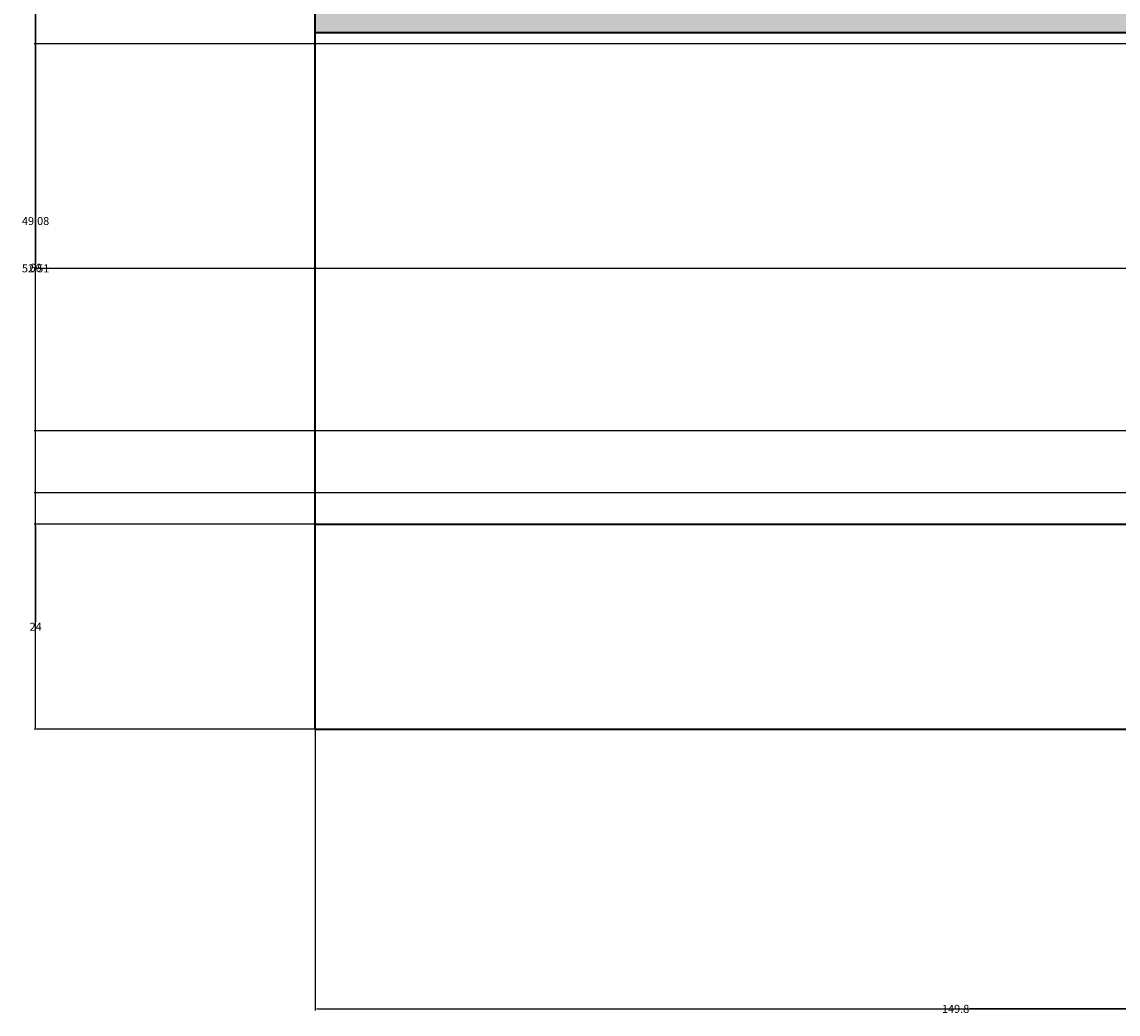
# Model space of a CAD drawing. Units: inches. Extents: x -5 to 714, y 84 to 644.
# Tile 1 of 20: x -4 to 124, y 84 to 200. Entities that reach past the tile are written whole.
import ezdxf

# ---------------------------------------------------------------- set-up
doc = ezdxf.new("R2010")
doc.units = ezdxf.units.IN
doc.header["$MEASUREMENT"] = 0
for name, color, linetype, lineweight in [('A-ANNO-DIMS', 2, 'Continuous', 18), ('A-ELEV', 7, 'Continuous', 35), ('A-ELEV-PATT', 8, 'Continuous', 13)]:
    doc.layers.add(name, color=color, linetype=linetype, lineweight=lineweight)
doc.styles.get("Standard").update_dxf_attribs({"font": 'arial.ttf'})
doc.dimstyles.get("Standard").update_dxf_attribs({"dimtxt": 0.9375, "dimasz": 0.18, "dimexe": 0.18, "dimexo": 0.0625, "dimgap": 0.09, "dimtad": 0, "dimtih": 1, "dimtoh": 1, "dimdec": 4, "dimzin": 0, "dimdsep": 46, "dimlunit": 4, "dimtxsty": 'Standard', "dimcen": 0.09, "dimadec": 0, "dimazin": 0, "dimtfac": 1, "dimtdec": 4, "dimtofl": 0, "dimtmove": 0, "dimatfit": 3, "dimfxl": 1, "dimtolj": 1, "dimtzin": 0, "dimarcsym": 0})

# ---------------------------------------------------------------- blocks, each defined once
blk = doc.blocks.new('*D1')
at = {"layer": 'A-ANNO-DIMS', "color": 0, "lineweight": -2, "transparency": 16777216}
for p, q in [((30.14, 117.13), (30.14, 84.31)), ((679.78, 117.13), (679.78, 84.31)), ((30.32, 84.49), (353.29, 84.49)), ((679.6, 84.49), (356.64, 84.49))]:
    blk.add_line(p, q, dxfattribs=at)
at = {"layer": 'A-ANNO-DIMS', "color": 0, "transparency": 16777216}
for points in [[(30.32, 84.52), (30.32, 84.46), (30.14, 84.49)], [(679.6, 84.52), (679.6, 84.46), (679.78, 84.49)]]:
    blk.add_solid(points, dxfattribs=at)
at = {"layer": 'Defpoints', "color": 0, "transparency": 16777216}
for p in [(30.14, 117.19), (679.78, 117.19), (679.78, 84.49)]:
    blk.add_point(p, dxfattribs=at)
at = {"layer": 'A-ANNO-DIMS', "color": 0, "transparency": 16777216, "insert": (354.96, 84.49), "char_height": 0.938, "attachment_point": 5}
blk.add_mtext('\\A1;649.6', dxfattribs=at)
blk = doc.blocks.new('*D2')
at = {"layer": 'A-ANNO-DIMS', "color": 0, "lineweight": -2, "transparency": 16777216}
for p, q in [((67.93, 610.73), (-2.74, 610.73)), ((-2.56, 610.55), (-2.56, 364.53)), ((-2.56, 117.37), (-2.56, 363.39)), ((30.08, 117.19), (-2.74, 117.19))]:
    blk.add_line(p, q, dxfattribs=at)
at = {"layer": 'A-ANNO-DIMS', "color": 0, "transparency": 16777216}
for points in [[(-2.59, 610.55), (-2.53, 610.55), (-2.56, 610.73)], [(-2.59, 117.37), (-2.53, 117.37), (-2.56, 117.19)]]:
    blk.add_solid(points, dxfattribs=at)
at = {"layer": 'Defpoints', "color": 0, "transparency": 16777216}
for p in [(-2.56, 610.73), (67.99, 610.73), (30.14, 117.19)]:
    blk.add_point(p, dxfattribs=at)
at = {"layer": 'A-ANNO-DIMS', "color": 0, "transparency": 16777216, "insert": (-2.56, 363.96), "char_height": 0.938, "attachment_point": 5}
blk.add_mtext('\\A1;493.5', dxfattribs=at)
blk = doc.blocks.new('*D3')
at = {"layer": 'A-ANNO-DIMS', "color": 0, "lineweight": -2, "transparency": 16777216}
for p, q in [((30.08, 141.19), (-2.74, 141.19)), ((-2.56, 141.01), (-2.56, 129.75)), ((-2.56, 117.37), (-2.56, 128.63)), ((30.08, 117.19), (-2.74, 117.19))]:
    blk.add_line(p, q, dxfattribs=at)
at = {"layer": 'A-ANNO-DIMS', "color": 0, "transparency": 16777216}
for points in [[(-2.59, 141.01), (-2.53, 141.01), (-2.56, 141.19)], [(-2.59, 117.37), (-2.53, 117.37), (-2.56, 117.19)]]:
    blk.add_solid(points, dxfattribs=at)
at = {"layer": 'Defpoints', "color": 0, "transparency": 16777216}
for p in [(-2.56, 141.19), (30.14, 141.19), (30.14, 117.19)]:
    blk.add_point(p, dxfattribs=at)
at = {"layer": 'A-ANNO-DIMS', "color": 0, "transparency": 16777216, "insert": (-2.56, 129.19), "char_height": 0.938, "attachment_point": 5}
blk.add_mtext('\\A1;24', dxfattribs=at)
blk = doc.blocks.new('*D4')
at = {"layer": 'A-ANNO-DIMS', "color": 0, "lineweight": -2, "transparency": 16777216}
for p, q in [((30.08, 201.19), (-2.74, 201.19)), ((-2.56, 201.01), (-2.56, 171.76)), ((-2.56, 141.37), (-2.56, 170.62)), ((30.08, 141.19), (-2.74, 141.19))]:
    blk.add_line(p, q, dxfattribs=at)
at = {"layer": 'A-ANNO-DIMS', "color": 0, "transparency": 16777216}
for points in [[(-2.59, 201.01), (-2.53, 201.01), (-2.56, 201.19)], [(-2.59, 141.37), (-2.53, 141.37), (-2.56, 141.19)]]:
    blk.add_solid(points, dxfattribs=at)
at = {"layer": 'Defpoints', "color": 0, "transparency": 16777216}
for p in [(-2.56, 201.19), (30.14, 201.19), (30.14, 141.19)]:
    blk.add_point(p, dxfattribs=at)
at = {"layer": 'A-ANNO-DIMS', "color": 0, "transparency": 16777216, "insert": (-2.56, 171.19), "char_height": 0.938, "attachment_point": 5}
blk.add_mtext('\\A1;60', dxfattribs=at)
blk = doc.blocks.new('*D65')
at = {"layer": 'A-ANNO-DIMS', "color": 0, "lineweight": -2, "transparency": 16777216}
for p, q in [((325.77, 266), (-2.74, 266)), ((-2.56, 265.82), (-2.56, 219.13)), ((-2.56, 171.3), (-2.56, 217.99)), ((325.77, 171.12), (-2.74, 171.12))]:
    blk.add_line(p, q, dxfattribs=at)
at = {"layer": 'A-ANNO-DIMS', "color": 0, "transparency": 16777216}
for points in [[(-2.59, 265.82), (-2.53, 265.82), (-2.56, 266)], [(-2.59, 171.3), (-2.53, 171.3), (-2.56, 171.12)]]:
    blk.add_solid(points, dxfattribs=at)
at = {"layer": 'Defpoints', "color": 0, "transparency": 16777216}
for p in [(-2.56, 266), (325.83, 266), (325.83, 171.12)]:
    blk.add_point(p, dxfattribs=at)
at = {"layer": 'A-ANNO-DIMS', "color": 0, "transparency": 16777216, "insert": (-2.56, 218.56), "char_height": 0.938, "attachment_point": 5}
blk.add_mtext('\\A1;94.88', dxfattribs=at)
blk = doc.blocks.new('*D73')
at = {"layer": 'A-ANNO-DIMS', "color": 0, "lineweight": -2, "transparency": 16777216}
for p, q in [((30.14, 141.13), (30.14, 84.31)), ((179.93, 141.13), (179.93, 84.31)), ((30.32, 84.49), (103.41, 84.49)), ((179.75, 84.49), (106.67, 84.49))]:
    blk.add_line(p, q, dxfattribs=at)
at = {"layer": 'A-ANNO-DIMS', "color": 0, "transparency": 16777216}
for points in [[(30.32, 84.52), (30.32, 84.46), (30.14, 84.49)], [(179.75, 84.52), (179.75, 84.46), (179.93, 84.49)]]:
    blk.add_solid(points, dxfattribs=at)
at = {"layer": 'Defpoints', "color": 0, "transparency": 16777216}
for p in [(30.14, 141.19), (179.93, 141.19), (179.93, 84.49)]:
    blk.add_point(p, dxfattribs=at)
at = {"layer": 'A-ANNO-DIMS', "color": 0, "transparency": 16777216, "insert": (105.04, 84.49), "char_height": 0.938, "attachment_point": 5}
blk.add_mtext('\\A1;149.8', dxfattribs=at)
blk = doc.blocks.new('*D82')
at = {"layer": 'A-ANNO-DIMS', "color": 0, "lineweight": -2, "transparency": 16777216}
for p, q in [((263.37, 201.19), (-2.74, 201.19)), ((-2.56, 201.01), (-2.56, 177.22)), ((-2.56, 152.3), (-2.56, 176.09)), ((263.37, 152.12), (-2.74, 152.12))]:
    blk.add_line(p, q, dxfattribs=at)
at = {"layer": 'A-ANNO-DIMS', "color": 0, "transparency": 16777216}
for points in [[(-2.59, 201.01), (-2.53, 201.01), (-2.56, 201.19)], [(-2.59, 152.3), (-2.53, 152.3), (-2.56, 152.12)]]:
    blk.add_solid(points, dxfattribs=at)
at = {"layer": 'Defpoints', "color": 0, "transparency": 16777216}
for p in [(-2.56, 201.19), (263.43, 201.19), (263.43, 152.12)]:
    blk.add_point(p, dxfattribs=at)
at = {"layer": 'A-ANNO-DIMS', "color": 0, "transparency": 16777216, "insert": (-2.56, 176.66), "char_height": 0.938, "attachment_point": 5}
blk.add_mtext('\\A1;49.08', dxfattribs=at)
blk = doc.blocks.new('*D87')
at = {"layer": 'A-ANNO-DIMS', "color": 0, "lineweight": -2, "transparency": 16777216}
for p, q in [((306.9, 197.38), (-2.74, 197.38)), ((-2.56, 197.2), (-2.56, 171.69)), ((-2.56, 145.04), (-2.56, 170.55)), ((306.9, 144.86), (-2.74, 144.86))]:
    blk.add_line(p, q, dxfattribs=at)
at = {"layer": 'A-ANNO-DIMS', "color": 0, "transparency": 16777216}
for points in [[(-2.59, 197.2), (-2.53, 197.2), (-2.56, 197.38)], [(-2.59, 145.04), (-2.53, 145.04), (-2.56, 144.86)]]:
    blk.add_solid(points, dxfattribs=at)
at = {"layer": 'Defpoints', "color": 0, "transparency": 16777216}
for p in [(-2.56, 197.38), (306.96, 197.38), (306.96, 144.86)]:
    blk.add_point(p, dxfattribs=at)
at = {"layer": 'A-ANNO-DIMS', "color": 0, "transparency": 16777216, "insert": (-2.56, 171.12), "char_height": 0.938, "attachment_point": 5}
blk.add_mtext('\\A1;52.51', dxfattribs=at)
blk = doc.blocks.new('*D89')
at = {"layer": 'A-ANNO-DIMS', "color": 0, "lineweight": -2, "transparency": 16777216}
for p, q in [((541.31, 197.38), (-2.74, 197.38)), ((-2.56, 197.2), (-2.56, 171.69)), ((-2.56, 145.04), (-2.56, 170.55)), ((541.31, 144.86), (-2.74, 144.86))]:
    blk.add_line(p, q, dxfattribs=at)
at = {"layer": 'A-ANNO-DIMS', "color": 0, "transparency": 16777216}
for points in [[(-2.59, 197.2), (-2.53, 197.2), (-2.56, 197.38)], [(-2.59, 145.04), (-2.53, 145.04), (-2.56, 144.86)]]:
    blk.add_solid(points, dxfattribs=at)
at = {"layer": 'Defpoints', "color": 0, "transparency": 16777216}
for p in [(-2.56, 197.38), (541.38, 197.38), (541.38, 144.86)]:
    blk.add_point(p, dxfattribs=at)
at = {"layer": 'A-ANNO-DIMS', "color": 0, "transparency": 16777216, "insert": (-2.56, 171.12), "char_height": 0.938, "attachment_point": 5}
blk.add_mtext('\\A1;52.51', dxfattribs=at)

msp = doc.modelspace()

# ---------------------------------------------------------------- hatches: boundary and pattern name
at = {"layer": 'A-ELEV-PATT', "transparency": 33554687}
h = msp.add_hatch(color=256, dxfattribs=at)
h.dxf.hatch_style = 1
h.paths.add_polyline_path([(188.3677, 525.1928), (67.9893, 525.1928), (67.9893, 489.1928), (67.9893, 345.1928), (126.7303, 345.1928), (126.7303, 480.1709), (229.3575, 480.1709), (229.3575, 525.1928), (212.6043, 525.1928), (212.6043, 482.7164), (211.0019, 482.7164), (211.0019, 525.1928), (207.6919, 525.1928), (199.9852, 525.1928), (199.9852, 482.7164), (198.3828, 482.7164), (198.3828, 525.1928), (189.9701, 525.1928), (189.9701, 482.7164), (188.3677, 482.7164)])
h.paths.add_polyline_path([(121.3589, 336.2066), (75.5048, 336.2066), (75.5048, 319.345), (121.3589, 319.345)])
h.paths.add_polyline_path([(121.3589, 319.345), (75.5048, 319.345), (75.5048, 302.3045), (121.3589, 302.3045)])
h.paths.add_polyline_path([(121.3589, 302.3045), (75.5048, 302.3045), (75.5048, 282.8561), (121.3589, 282.8561)])
h.paths.add_polyline_path([(121.3589, 282.8561), (75.5048, 282.8561), (75.5048, 261.5556), (121.3589, 261.5556)])
h.paths.add_polyline_path([(121.3589, 261.5556), (75.5048, 261.5556), (75.5048, 243.7009), (121.3589, 243.7009)])
h.paths.add_polyline_path([(121.3589, 243.7009), (75.5048, 243.7009), (75.5048, 223.5117), (121.3589, 223.5117)])
h.paths.add_polyline_path([(121.3589, 223.5117), (75.5048, 223.5117), (75.5048, 212.5836), (121.3589, 212.5836)])
h.paths.add_polyline_path([(121.3589, 212.5836), (75.5048, 212.5836), (75.5048, 201.1928), (121.3589, 201.1928)])
h.paths.add_polyline_path([(179.9335, 201.1928), (30.1395, 201.1928), (30.1395, 198.7054), (179.9335, 198.7054)])
h.paths.add_polyline_path([(187.6349, 201.1928), (179.9335, 201.1928), (179.9335, 198.7054), (179.9335, 141.1928), (269.2446, 141.1928), (269.2446, 201.1928), (263.4349, 201.1928), (263.4349, 152.1176), (187.6349, 152.1176)])
h.paths.add_polyline_path([(269.2446, 277.0513), (269.2446, 287.501), (269.2446, 306.6286), (578.0915, 306.6286), (578.0915, 201.1928), (593.428, 201.1928), (593.428, 315.0968), (584.4202, 315.0968), (259.0665, 315.0968), (259.0665, 201.1928), (263.4349, 201.1928), (269.2446, 201.1928)])

# ---------------------------------------------------------------- linework, layer by layer
at = {"layer": 'A-ELEV'}
for p, q in [((30.1395, 141.1928), (30.1395, 201.1928)), ((30.1395, 198.7054), (179.9335, 198.7054)), ((30.1395, 117.1928), (30.1395, 141.1928)), ((30.1395, 141.1928), (548.9353, 141.1928)), ((30.1395, 117.1928), (548.9353, 117.1928))]:
    msp.add_line(p, q, dxfattribs=at)

# ---------------------------------------------------------------- dimensions: what is measured, and where the dimension line sits
at = {"layer": 'A-ANNO-DIMS'}
for base, p1, p2, override, picture, middle in [((-2.5605, 610.7276), (30.1395, 117.1928), (67.9893, 610.7276), {"dimdec": 1, "dimlfac": 1, "dimrnd": 0, "dimzin": 0, "dimdsep": 46, "dimlunit": 2}, '*D2', (-2.5605, 363.9602)), ((-2.5605, 266.0021), (325.8305, 171.1197), (325.8305, 266.0021), {"dimdec": 2, "dimlfac": 1, "dimrnd": 0, "dimzin": 0, "dimdsep": 46, "dimlunit": 2}, '*D65', (-2.5605, 218.5609)), ((-2.5605, 201.1928), (263.4349, 152.1176), (263.4349, 201.1928), {"dimdec": 2, "dimlfac": 1, "dimrnd": 0, "dimzin": 0, "dimdsep": 46, "dimlunit": 2}, '*D82', (-2.5605, 176.6552)), ((-2.5605, 201.1928), (30.1395, 141.1928), (30.1395, 201.1928), {"dimdec": 0, "dimlfac": 1, "dimrnd": 0, "dimzin": 0, "dimdsep": 46, "dimlunit": 2}, '*D4', (-2.5605, 171.1928)), ((-2.5605, 197.3754), (306.958, 144.8639), (306.958, 197.3754), {"dimdec": 2, "dimlfac": 1, "dimrnd": 0, "dimzin": 0, "dimdsep": 46, "dimlunit": 2}, '*D87', (-2.5605, 171.1197)), ((-2.5605, 197.3754), (541.3773, 144.8639), (541.3773, 197.3754), {"dimdec": 2, "dimlfac": 1, "dimrnd": 0, "dimzin": 0, "dimdsep": 46, "dimlunit": 2}, '*D89', (-2.5605, 171.1197)), ((-2.5605, 141.1928), (30.1395, 117.1928), (30.1395, 141.1928), {"dimdec": 0, "dimlfac": 1, "dimrnd": 0, "dimzin": 0, "dimdsep": 46, "dimlunit": 2}, '*D3', (-2.5605, 129.1928))]:
    dim = msp.add_linear_dim(base=base, p1=p1, p2=p2, angle=90, dimstyle='Standard', override=override, dxfattribs=at)
    dim.commit()
    dim.dimension.update_dxf_attribs({"geometry": picture, "text_midpoint": middle})
for base, p1, p2, picture, middle in [((179.9335, 84.4928), (30.1395, 141.1928), (179.9335, 141.1928), '*D73', (105.0365, 84.4928)), ((679.7826, 84.4928), (30.1395, 117.1928), (679.7826, 117.1928), '*D1', (354.9611, 84.4928))]:
    dim = msp.add_linear_dim(base=base, p1=p1, p2=p2, dimstyle='Standard', override={"dimdec": 1, "dimlfac": 1, "dimrnd": 0, "dimzin": 0, "dimdsep": 46, "dimlunit": 2}, dxfattribs=at)
    dim.commit()
    dim.dimension.update_dxf_attribs({"geometry": picture, "text_midpoint": middle})

doc.saveas('drawing.dxf')
